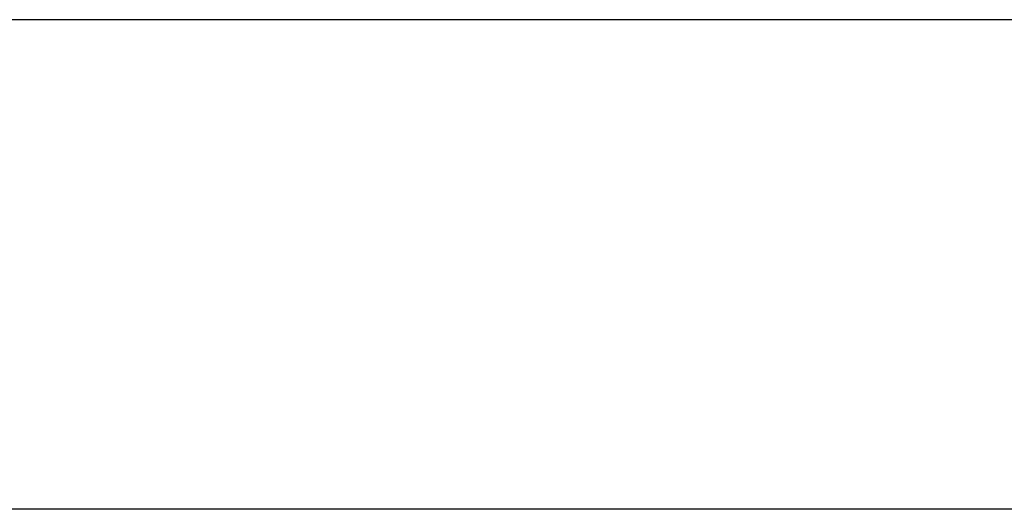
# Model space of a CAD drawing. Units: millimetres. Extents: x 0 to 2267, y 0 to 1823.
# Tile 3 of 256: x 1378 to 1459, y 1077 to 1117. Entities that reach past the tile are written whole.
import ezdxf

# ---------------------------------------------------------------- set-up
doc = ezdxf.new("R2010")
doc.units = ezdxf.units.MM
doc.header["$MEASUREMENT"] = 0
doc.layers.add('M-DIMS', color=2, linetype='Continuous', lineweight=25)
doc.styles.get("Standard").update_dxf_attribs({"font": 'arial.ttf'})
doc.dimstyles.get("Standard").update_dxf_attribs({"dimtxt": 7, "dimasz": 4, "dimexe": 0.18, "dimexo": 0.0625, "dimgap": 0.09, "dimtad": 0, "dimdec": 0, "dimzin": 0, "dimdsep": 46, "dimtxsty": 'Standard', "dimcen": 0.09, "dimadec": 0, "dimazin": 0, "dimtfac": 1, "dimtdec": 0, "dimtofl": 0, "dimtmove": 0, "dimatfit": 3, "dimfxl": 1, "dimtolj": 1, "dimtzin": 0, "dimarcsym": 0})

# ---------------------------------------------------------------- blocks, each defined once
blk = doc.blocks.new('*D9')
at = {"layer": 'Defpoints', "color": 0, "transparency": 16777216}
for p in [(1332.087, 1117.417), (1505.929, 1117.417), (1505.929, 1077.417)]:
    blk.add_point(p, dxfattribs=at)
at = {"layer": 'M-DIMS', "color": 0, "lineweight": -2, "transparency": 16777216}
for p, q in [((1505.866, 1117.417), (1331.907, 1117.417)), ((1332.087, 1113.417), (1332.087, 1102.65)), ((1332.087, 1081.417), (1332.087, 1092.184)), ((1505.866, 1077.417), (1331.907, 1077.417))]:
    blk.add_line(p, q, dxfattribs=at)
at = {"layer": 'M-DIMS', "color": 0, "transparency": 16777216}
for points in [[(1331.42, 1113.417), (1332.753, 1113.417), (1332.087, 1117.417)], [(1331.42, 1081.417), (1332.753, 1081.417), (1332.087, 1077.417)]]:
    blk.add_solid(points, dxfattribs=at)
at = {"layer": 'M-DIMS', "color": 0, "transparency": 16777216, "insert": (1332.087, 1097.417), "char_height": 7, "attachment_point": 5, "rotation": 90}
blk.add_mtext('\\A1;40', dxfattribs=at)
blk = doc.blocks.new('*D10')
at = {"layer": 'Defpoints', "color": 0, "transparency": 16777216}
for p in [(1332.087, 1287.766), (1505.929, 1287.766), (1505.929, 1117.417)]:
    blk.add_point(p, dxfattribs=at)
at = {"layer": 'M-DIMS', "color": 0, "lineweight": -2, "transparency": 16777216}
for p, q in [((1505.866, 1287.766), (1331.907, 1287.766)), ((1332.087, 1283.766), (1332.087, 1216.908)), ((1332.087, 1121.417), (1332.087, 1188.275)), ((1505.866, 1117.417), (1331.907, 1117.417))]:
    blk.add_line(p, q, dxfattribs=at)
at = {"layer": 'M-DIMS', "color": 0, "transparency": 16777216}
for points in [[(1331.42, 1283.766), (1332.753, 1283.766), (1332.087, 1287.766)], [(1331.42, 1121.417), (1332.753, 1121.417), (1332.087, 1117.417)]]:
    blk.add_solid(points, dxfattribs=at)
at = {"layer": 'M-DIMS', "color": 0, "transparency": 16777216, "insert": (1332.087, 1202.591), "char_height": 7, "attachment_point": 5, "rotation": 90}
blk.add_mtext('\\A1;170.35', dxfattribs=at)

msp = doc.modelspace()

# ---------------------------------------------------------------- dimensions: what is measured, and where the dimension line sits
at = {"layer": 'M-DIMS'}
for base, p1, p2, override, picture, middle in [((1332.087, 1287.766), (1505.929, 1117.417), (1505.929, 1287.766), {"dimdec": 2, "dimlfac": 1, "dimrnd": 0, "dimzin": 0, "dimdsep": 46, "dimlunit": 2}, '*D10', (1332.087, 1202.591)), ((1332.087, 1117.417), (1505.929, 1077.417), (1505.929, 1117.417), {"dimdec": 0, "dimlfac": 1, "dimrnd": 0, "dimzin": 0, "dimdsep": 46, "dimlunit": 2}, '*D9', (1332.087, 1097.417))]:
    dim = msp.add_linear_dim(base=base, p1=p1, p2=p2, angle=90, dimstyle='Standard', override=override, dxfattribs=at)
    dim.commit()
    dim.dimension.update_dxf_attribs({"geometry": picture, "text_midpoint": middle})

doc.saveas('drawing.dxf')
